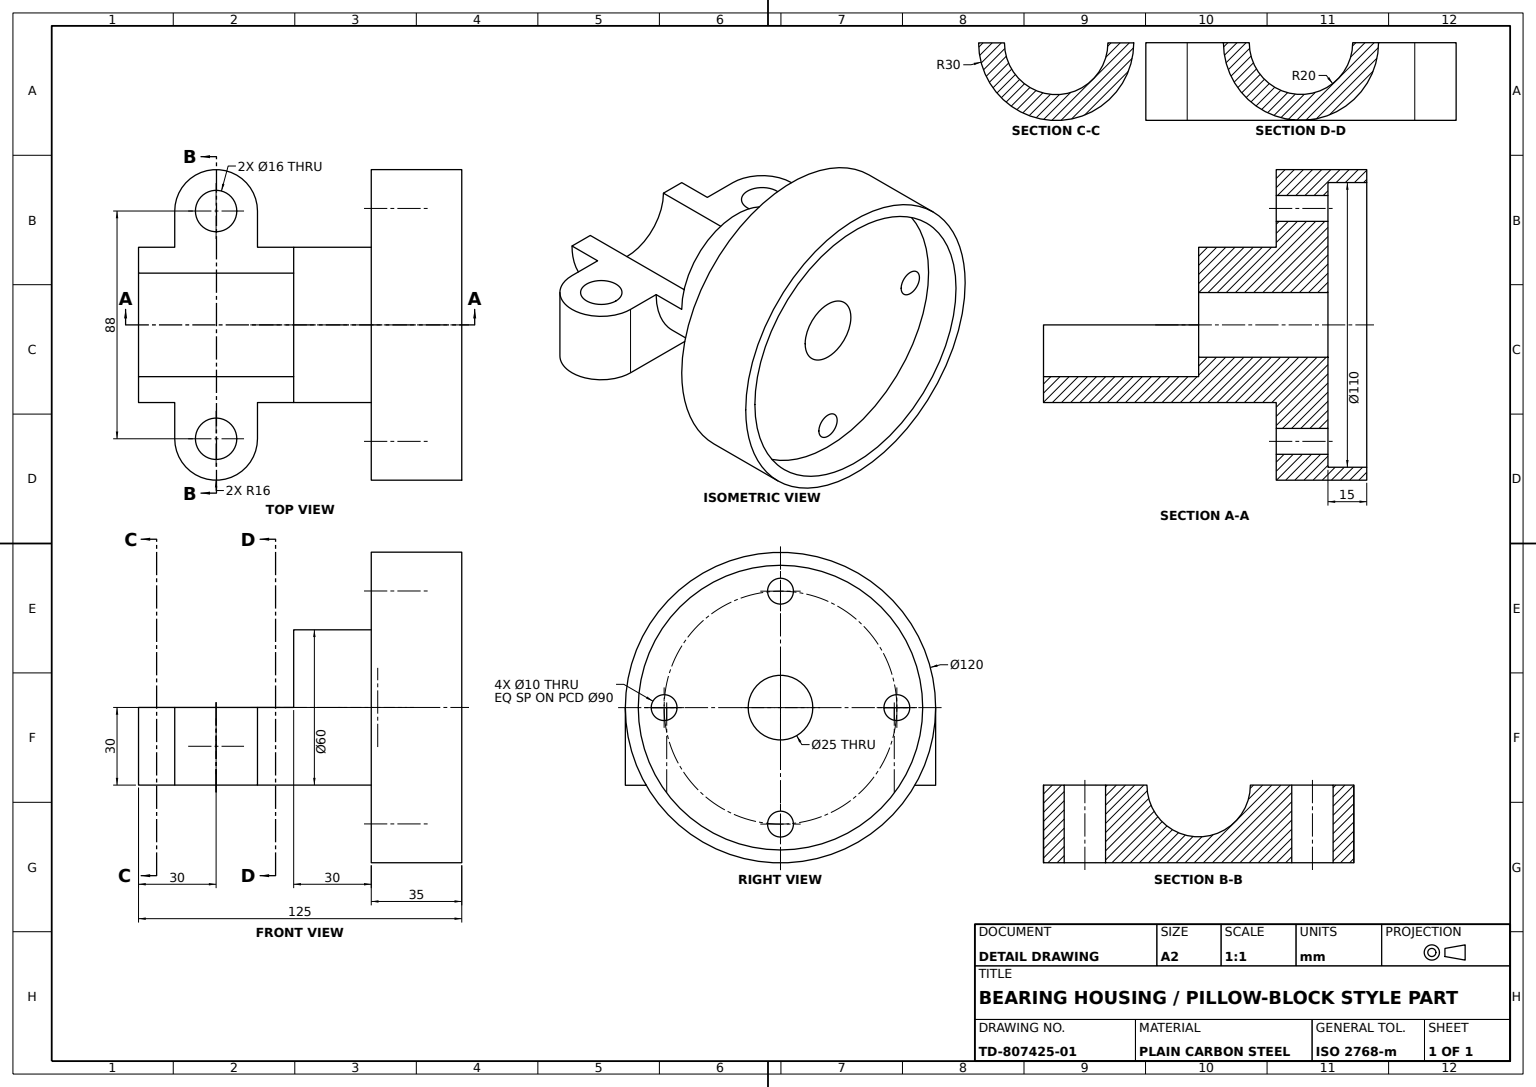
SolidWorks part; units mm, degrees
material "Plain Carbon Steel"
ref_plane "Front Plane" through (0, 0, 0) normal (0, 0, 1) x (1, 0, 0)
ref_plane "Top Plane" through (0, 0, 0) normal (0, 1, 0) x (1, 0, 0)
ref_plane "Right Plane" through (0, 0, 0) normal (1, 0, 0) x (0, 0, -1)
sketch "Flange Profile" plane through (0, 0, 0) normal (0, 0, 1) x (1, 0, 0)
  circle A0 centre (0, 0) radius 60
  dimension "D1" = 120
  dimension "D2" = 120
extrude "Flange Ø120" add sketch "Flange Profile" against normal blind 35
sketch "Hub Profile" plane through (0, 0, 0) normal (0, 0, 1) x (1, 0, 0)
  circle A0 centre (0, 0) radius 30
  dimension "D1" = 60
extrude "Hub" add sketch "Hub Profile" along normal blind 30
sketch "Saddle Profile" plane through (0, 0, 30) normal (0, 0, 1) x (1, 0, 0)
  line L0 (-30, 0) -> (30, 0)
  arc A0 (-30, 0) -> (30, 0) centre (0, 0) ccw
  dimension "D1" = 30
extrude "Half-Bearing Saddle" add sketch "Saddle Profile" along normal blind 60
sketch "Flange Recess Profile" plane through (0, 0, -35) normal (0, 0, -1) x (-1, 0, 0)
  circle A0 centre (0, 0) radius 55
  dimension "D1" = 110
  dimension "D2" = 110
extrude "Flange Recess Ø110" cut sketch "Flange Recess Profile" against normal blind 15
sketch "Flange Bolt Holes Profile" plane through (0, 0, 0) normal (0, 0, 1) x (1, 0, 0)
  circle A1 centre (45, 0) radius 5
  circle A2 centre (0, 45) radius 5
  circle A3 centre (-45, 0) radius 5
  circle A4 centre (0, -45) radius 5
  dimension "D1" = 10
  dimension "D2" = 45
  dimension "D3" = 45
  dimension "D4" = 45
  dimension "D5" = 45
extrude "Flange Bolt Holes" cut sketch "Flange Bolt Holes Profile" against normal blind 52
sketch "Saddle Bore Profile" plane through (0, 0, 90) normal (0, 0, 1) x (1, 0, 0)
  line L0 (-20, 0) -> (20, 0)
  arc A0 (-20, 0) -> (20, 0) centre (0, 0) ccw
  dimension "D1" = 20
  dimension "D2" = 40
extrude "Saddle Bore R20" cut sketch "Saddle Bore Profile" against normal blind 60
sketch "Shaft Bore Profile" plane through (0, 0, 30) normal (0, 0, 1) x (1, 0, 0)
  circle A0 centre (0, 0) radius 12.5
  dimension "D1" = 25
  dimension "D2" = 25
extrude "Shaft Bore Ø25" cut sketch "Shaft Bore Profile" against normal blind 60
sketch "Mounting Lug A Profile" plane through (0, 0, 0) normal (0, 1, 0) x (1, 0, 0)
  line L0 (-44, -76) -> (-30, -76)
  line L1 (-20, -30) -> (-20, -90) construction
  line L3 (-30, -90) -> (-30, -30) construction
  line L6 (-30, -76) -> (-30, -44)
  line L7 (-30, -44) -> (-44, -44)
  arc A0 (-44, -44) -> (-44, -76) centre (-44, -60) ccw
  dimension "D1" = 16
  dimension "D2" = 24
  dimension "D3" = 30
extrude "Mounting Lug A" add sketch "Mounting Lug A Profile" against normal blind 30 separate body
sketch "Mounting Lug B Profile" plane through (0, 0, 0) normal (0, 1, 0) x (1, 0, 0)
  line L0 (20, -30) -> (20, -90) construction
  line L1 (30, -30) -> (20, -30) construction
  line L2 (44, -44) -> (30, -44)
  line L3 (30, -90) -> (30, -30) construction
  line L4 (30, -44) -> (30, -76)
  line L5 (30, -76) -> (44, -76)
  arc A0 (44, -76) -> (44, -44) centre (44, -60) ccw
  dimension "D1" = 16
  dimension "D2" = 24
  dimension "D3" = 30
extrude "Mounting Lug B" add sketch "Mounting Lug B Profile" against normal blind 30 separate body
sketch "Lug Bridge Profile" plane through (0, -30, 0) normal (0, -1, 0) x (1, 0, 0)
  line L0 (30, 76) -> (-30, 76)
  line L1 (-30, 76) -> (-30, 44)
  line L2 (-30, 44) -> (30, 44)
  line L3 (30, 44) -> (30, 76)
extrude "Lug Bridge" add sketch "Lug Bridge Profile" against normal blind 30
sketch "Bridge Relief Profile" plane through (0, 0, 76) normal (0, 0, 1) x (1, 0, 0)
  line L0 (-20, 0) -> (20, 0)
  arc A0 (-20, 0) -> (20, 0) centre (0, 0) ccw
extrude "Bridge Bore Relief" cut sketch "Bridge Relief Profile" against normal blind 35
sketch "Lug Holes Profile" plane through (0, 0, 0) normal (0, 1, 0) x (1, 0, 0)
  circle A0 centre (-44, -60) radius 8
  circle A1 centre (44, -60) radius 8
  dimension "D1" = 16
  dimension "D2" = 16
  dimension "D3" = 16
extrude "Lug Holes 2xØ16" cut sketch "Lug Holes Profile" against normal blind 35
